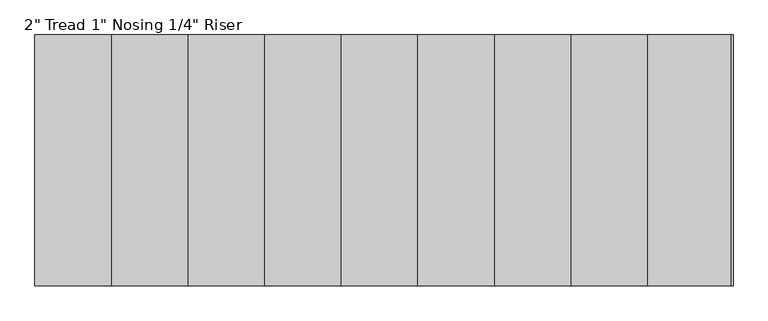
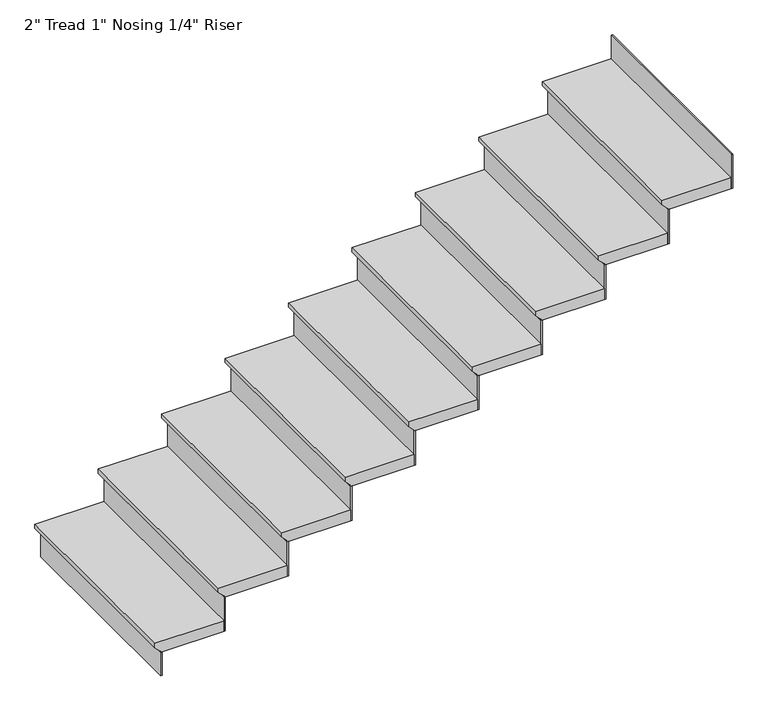
"""IFC4 building model written with IfcOpenShell, lengths in millimetres: stair flight geometry."""

from ifc_helpers import new_model, si_unit, origin, place, context, project, spatial, faceted_brep, source, transform, mapped, element, save


def stair_flight_45c7a08f(model_context):
    return source(origin(), model_context, "Body", "Brep", [
        faceted_brep([(-1591.1154463, -4737.3544725, 12942.57), (-1591.1154463, -4737.3544725, 12961.62), (-1591.1154463, -3822.9544725, 12961.62), (-1591.1154463, -3822.9544725, 12942.57), (-1565.7154463, -4737.3544725, 12917.17), (-1565.7154463, -3822.9544725, 12917.17), (-1286.3154463, -4737.3544725, 12961.62), (-1286.3154463, -3822.9544725, 12961.62), (-1565.7154463, -3822.9544725, 12910.82), (-1286.3154463, -3822.9544725, 12910.82), (-1286.3154463, -4737.3544725, 12910.82), (-1565.7154463, -4737.3544725, 12910.82)], [[[0, 1, 2, 3]], [[4, 0, 3, 5]], [[2, 1, 6, 7]], [[8, 9, 10, 11]], [[2, 7, 9, 8, 5, 3]], [[8, 11, 4, 5]], [[6, 1, 0, 4, 11, 10]], [[7, 6, 10, 9]]]),
        faceted_brep([(-1565.7154463, -4737.3544725, 12910.82), (-1565.7154463, -4737.3544725, 12801.6), (-1559.3654463, -4737.3544725, 12801.6), (-1559.3654463, -4737.3544725, 12910.82), (-1565.7154463, -3822.9544725, 12910.82), (-1559.3654463, -3822.9544725, 12910.82), (-1559.3654463, -3822.9544725, 12801.6), (-1565.7154463, -3822.9544725, 12801.6)], [[[0, 1, 2, 3]], [[4, 5, 6, 7]], [[1, 0, 4, 7]], [[2, 1, 7, 6]], [[3, 2, 6, 5]], [[0, 3, 5, 4]]]),
        faceted_brep([(-1286.3154463, -4737.3544725, 13070.84), (-1286.3154463, -4737.3544725, 12910.82), (-1279.9654463, -4737.3544725, 12910.82), (-1279.9654463, -4737.3544725, 13070.84), (-1286.3154463, -3822.9544725, 13070.84), (-1279.9654463, -3822.9544725, 13070.84), (-1279.9654463, -3822.9544725, 12910.82), (-1286.3154463, -3822.9544725, 12910.82)], [[[0, 1, 2, 3]], [[4, 5, 6, 7]], [[1, 0, 4, 7]], [[2, 1, 7, 6]], [[3, 2, 6, 5]], [[0, 3, 5, 4]]]),
        faceted_brep([(-1311.7154463, -3822.9544725, 13121.64), (-1311.7154463, -4737.3544725, 13121.64), (-1006.9154463, -4737.3544725, 13121.64), (-1006.9154463, -3822.9544725, 13121.64), (-1286.3154463, -3822.9544725, 13070.84), (-1006.9154463, -3822.9544725, 13070.84), (-1006.9154463, -4737.3544725, 13070.84), (-1286.3154463, -4737.3544725, 13070.84), (-1286.3154463, -3822.9544725, 13077.19), (-1311.7154463, -3822.9544725, 13102.59), (-1286.3154463, -4737.3544725, 13077.19), (-1311.7154463, -4737.3544725, 13102.59)], [[[0, 1, 2, 3]], [[4, 5, 6, 7]], [[0, 3, 5, 4, 8, 9]], [[4, 7, 10, 8]], [[2, 1, 11, 10, 7, 6]], [[3, 2, 6, 5]], [[11, 1, 0, 9]], [[10, 11, 9, 8]]]),
        faceted_brep([(-1006.9154463, -4737.3544725, 13230.86), (-1006.9154463, -4737.3544725, 13070.84), (-1000.5654463, -4737.3544725, 13070.84), (-1000.5654463, -4737.3544725, 13230.86), (-1006.9154463, -3822.9544725, 13230.86), (-1000.5654463, -3822.9544725, 13230.86), (-1000.5654463, -3822.9544725, 13070.84), (-1006.9154463, -3822.9544725, 13070.84)], [[[0, 1, 2, 3]], [[4, 5, 6, 7]], [[1, 0, 4, 7]], [[2, 1, 7, 6]], [[3, 2, 6, 5]], [[0, 3, 5, 4]]]),
        faceted_brep([(-1032.3154463, -3822.9544725, 13281.66), (-1032.3154463, -4737.3544725, 13281.66), (-727.5154463, -4737.3544725, 13281.66), (-727.5154463, -3822.9544725, 13281.66), (-1006.9154463, -3822.9544725, 13230.86), (-727.5154463, -3822.9544725, 13230.86), (-727.5154463, -4737.3544725, 13230.86), (-1006.9154463, -4737.3544725, 13230.86), (-1006.9154463, -3822.9544725, 13237.21), (-1032.3154463, -3822.9544725, 13262.61), (-1006.9154463, -4737.3544725, 13237.21), (-1032.3154463, -4737.3544725, 13262.61)], [[[0, 1, 2, 3]], [[4, 5, 6, 7]], [[0, 3, 5, 4, 8, 9]], [[4, 7, 10, 8]], [[2, 1, 11, 10, 7, 6]], [[3, 2, 6, 5]], [[11, 1, 0, 9]], [[10, 11, 9, 8]]]),
        faceted_brep([(-727.5154463, -4737.3544725, 13390.88), (-727.5154463, -4737.3544725, 13230.86), (-721.1654463, -4737.3544725, 13230.86), (-721.1654463, -4737.3544725, 13390.88), (-727.5154463, -3822.9544725, 13390.88), (-721.1654463, -3822.9544725, 13390.88), (-721.1654463, -3822.9544725, 13230.86), (-727.5154463, -3822.9544725, 13230.86)], [[[0, 1, 2, 3]], [[4, 5, 6, 7]], [[1, 0, 4, 7]], [[2, 1, 7, 6]], [[3, 2, 6, 5]], [[0, 3, 5, 4]]]),
        faceted_brep([(-752.9154463, -3822.9544725, 13441.68), (-752.9154463, -4737.3544725, 13441.68), (-448.1154463, -4737.3544725, 13441.68), (-448.1154463, -3822.9544725, 13441.68), (-727.5154463, -3822.9544725, 13390.88), (-448.1154463, -3822.9544725, 13390.88), (-448.1154463, -4737.3544725, 13390.88), (-727.5154463, -4737.3544725, 13390.88), (-727.5154463, -3822.9544725, 13397.23), (-752.9154463, -3822.9544725, 13422.63), (-727.5154463, -4737.3544725, 13397.23), (-752.9154463, -4737.3544725, 13422.63)], [[[0, 1, 2, 3]], [[4, 5, 6, 7]], [[0, 3, 5, 4, 8, 9]], [[4, 7, 10, 8]], [[2, 1, 11, 10, 7, 6]], [[3, 2, 6, 5]], [[11, 1, 0, 9]], [[10, 11, 9, 8]]]),
        faceted_brep([(-448.1154463, -4737.3544725, 13550.9), (-448.1154463, -4737.3544725, 13390.88), (-441.7654463, -4737.3544725, 13390.88), (-441.7654463, -4737.3544725, 13550.9), (-448.1154463, -3822.9544725, 13550.9), (-441.7654463, -3822.9544725, 13550.9), (-441.7654463, -3822.9544725, 13390.88), (-448.1154463, -3822.9544725, 13390.88)], [[[0, 1, 2, 3]], [[4, 5, 6, 7]], [[1, 0, 4, 7]], [[2, 1, 7, 6]], [[3, 2, 6, 5]], [[0, 3, 5, 4]]]),
        faceted_brep([(-473.5154463, -3822.9544725, 13601.7), (-473.5154463, -4737.3544725, 13601.7), (-168.7154463, -4737.3544725, 13601.7), (-168.7154463, -3822.9544725, 13601.7), (-448.1154463, -3822.9544725, 13550.9), (-168.7154463, -3822.9544725, 13550.9), (-168.7154463, -4737.3544725, 13550.9), (-448.1154463, -4737.3544725, 13550.9), (-448.1154463, -3822.9544725, 13557.25), (-473.5154463, -3822.9544725, 13582.65), (-448.1154463, -4737.3544725, 13557.25), (-473.5154463, -4737.3544725, 13582.65)], [[[0, 1, 2, 3]], [[4, 5, 6, 7]], [[0, 3, 5, 4, 8, 9]], [[4, 7, 10, 8]], [[2, 1, 11, 10, 7, 6]], [[3, 2, 6, 5]], [[11, 1, 0, 9]], [[10, 11, 9, 8]]]),
        faceted_brep([(-168.7154463, -4737.3544725, 13710.92), (-168.7154463, -4737.3544725, 13550.9), (-162.3654463, -4737.3544725, 13550.9), (-162.3654463, -4737.3544725, 13710.92), (-168.7154463, -3822.9544725, 13710.92), (-162.3654463, -3822.9544725, 13710.92), (-162.3654463, -3822.9544725, 13550.9), (-168.7154463, -3822.9544725, 13550.9)], [[[0, 1, 2, 3]], [[4, 5, 6, 7]], [[1, 0, 4, 7]], [[2, 1, 7, 6]], [[3, 2, 6, 5]], [[0, 3, 5, 4]]]),
        faceted_brep([(-194.1154463, -3822.9544725, 13761.72), (-194.1154463, -4737.3544725, 13761.72), (110.6845537, -4737.3544725, 13761.72), (110.6845537, -3822.9544725, 13761.72), (-168.7154463, -3822.9544725, 13710.92), (110.6845537, -3822.9544725, 13710.92), (110.6845537, -4737.3544725, 13710.92), (-168.7154463, -4737.3544725, 13710.92), (-168.7154463, -3822.9544725, 13717.27), (-194.1154463, -3822.9544725, 13742.67), (-168.7154463, -4737.3544725, 13717.27), (-194.1154463, -4737.3544725, 13742.67)], [[[0, 1, 2, 3]], [[4, 5, 6, 7]], [[0, 3, 5, 4, 8, 9]], [[4, 7, 10, 8]], [[2, 1, 11, 10, 7, 6]], [[3, 2, 6, 5]], [[11, 1, 0, 9]], [[10, 11, 9, 8]]]),
        faceted_brep([(110.6845537, -4737.3544725, 13870.94), (110.6845537, -4737.3544725, 13710.92), (117.0345537, -4737.3544725, 13710.92), (117.0345537, -4737.3544725, 13870.94), (110.6845537, -3822.9544725, 13870.94), (117.0345537, -3822.9544725, 13870.94), (117.0345537, -3822.9544725, 13710.92), (110.6845537, -3822.9544725, 13710.92)], [[[0, 1, 2, 3]], [[4, 5, 6, 7]], [[1, 0, 4, 7]], [[2, 1, 7, 6]], [[3, 2, 6, 5]], [[0, 3, 5, 4]]]),
        faceted_brep([(85.2845537, -3822.9544725, 13921.74), (85.2845537, -4737.3544725, 13921.74), (390.0845537, -4737.3544725, 13921.74), (390.0845537, -3822.9544725, 13921.74), (110.6845537, -3822.9544725, 13870.94), (390.0845537, -3822.9544725, 13870.94), (390.0845537, -4737.3544725, 13870.94), (110.6845537, -4737.3544725, 13870.94), (110.6845537, -3822.9544725, 13877.29), (85.2845537, -3822.9544725, 13902.69), (110.6845537, -4737.3544725, 13877.29), (85.2845537, -4737.3544725, 13902.69)], [[[0, 1, 2, 3]], [[4, 5, 6, 7]], [[0, 3, 5, 4, 8, 9]], [[4, 7, 10, 8]], [[2, 1, 11, 10, 7, 6]], [[3, 2, 6, 5]], [[11, 1, 0, 9]], [[10, 11, 9, 8]]]),
        faceted_brep([(390.0845537, -4737.3544725, 14030.96), (390.0845537, -4737.3544725, 13870.94), (396.4345537, -4737.3544725, 13870.94), (396.4345537, -4737.3544725, 14030.96), (390.0845537, -3822.9544725, 14030.96), (396.4345537, -3822.9544725, 14030.96), (396.4345537, -3822.9544725, 13870.94), (390.0845537, -3822.9544725, 13870.94)], [[[0, 1, 2, 3]], [[4, 5, 6, 7]], [[1, 0, 4, 7]], [[2, 1, 7, 6]], [[3, 2, 6, 5]], [[0, 3, 5, 4]]]),
        faceted_brep([(364.6845537, -3822.9544725, 14081.76), (364.6845537, -4737.3544725, 14081.76), (669.4845537, -4737.3544725, 14081.76), (669.4845537, -3822.9544725, 14081.76), (390.0845537, -3822.9544725, 14030.96), (669.4845537, -3822.9544725, 14030.96), (669.4845537, -4737.3544725, 14030.96), (390.0845537, -4737.3544725, 14030.96), (390.0845537, -3822.9544725, 14037.31), (364.6845537, -3822.9544725, 14062.71), (390.0845537, -4737.3544725, 14037.31), (364.6845537, -4737.3544725, 14062.71)], [[[0, 1, 2, 3]], [[4, 5, 6, 7]], [[0, 3, 5, 4, 8, 9]], [[4, 7, 10, 8]], [[2, 1, 11, 10, 7, 6]], [[3, 2, 6, 5]], [[11, 1, 0, 9]], [[10, 11, 9, 8]]]),
        faceted_brep([(948.8845537, -4737.3544725, 14351.0), (948.8845537, -4737.3544725, 14190.98), (955.2345537, -4737.3544725, 14190.98), (955.2345537, -4737.3544725, 14351.0), (948.8845537, -3822.9544725, 14351.0), (955.2345537, -3822.9544725, 14351.0), (955.2345537, -3822.9544725, 14190.98), (948.8845537, -3822.9544725, 14190.98)], [[[0, 1, 2, 3]], [[4, 5, 6, 7]], [[1, 0, 4, 7]], [[2, 1, 7, 6]], [[3, 2, 6, 5]], [[0, 3, 5, 4]]]),
        faceted_brep([(669.4845537, -4737.3544725, 14190.98), (669.4845537, -4737.3544725, 14030.96), (675.8345537, -4737.3544725, 14030.96), (675.8345537, -4737.3544725, 14190.98), (669.4845537, -3822.9544725, 14190.98), (675.8345537, -3822.9544725, 14190.98), (675.8345537, -3822.9544725, 14030.96), (669.4845537, -3822.9544725, 14030.96)], [[[0, 1, 2, 3]], [[4, 5, 6, 7]], [[1, 0, 4, 7]], [[2, 1, 7, 6]], [[3, 2, 6, 5]], [[0, 3, 5, 4]]]),
        faceted_brep([(948.8845537, -3822.9544725, 14241.78), (923.4845537, -3822.9544725, 14241.78), (644.0845537, -3822.9544725, 14241.78), (644.0845537, -4737.3544725, 14241.78), (948.8845537, -4737.3544725, 14241.78), (923.4845537, -3822.9544725, 14190.98), (948.8845537, -3822.9544725, 14190.98), (948.8845537, -4737.3544725, 14190.98), (669.4845537, -4737.3544725, 14190.98), (669.4845537, -3822.9544725, 14190.98), (669.4845537, -3822.9544725, 14197.33), (644.0845537, -3822.9544725, 14222.73), (669.4845537, -4737.3544725, 14197.33), (644.0845537, -4737.3544725, 14222.73)], [[[0, 1, 2, 3, 4]], [[5, 6, 7, 8, 9]], [[1, 0, 6, 5]], [[2, 1, 5, 9, 10, 11]], [[9, 8, 12, 10]], [[4, 3, 13, 12, 8, 7]], [[0, 4, 7, 6]], [[13, 3, 2, 11]], [[12, 13, 11, 10]]]),
    ])


if __name__ == "__main__":
    model = new_model("IFC4")
    model_context = context("Model", 3, world=origin())
    ifc_project = project(units=[si_unit("LENGTHUNIT", "METRE", prefix="MILLI")], contexts=[model_context])
    site = spatial("IfcSite", under=ifc_project)
    building = spatial("IfcBuilding", under=site)
    placement = place(None, origin())
    stair_flight_shape = stair_flight_45c7a08f(model_context)
    element("IfcStairFlight", 1, ObjectType="2\" Tread 1\" Nosing 1/4\" Riser", at=placement, inside=building, context=model_context, shape_type="MappedRepresentation", body=[
        mapped(stair_flight_shape, transform((0.0, 0.0, 0.0), x_axis=(1.0, 0.0, 0.0), y_axis=(0.0, 1.0, 0.0), z_axis=(0.0, 0.0, 1.0))),
    ])
    save(model, "model.ifc")
